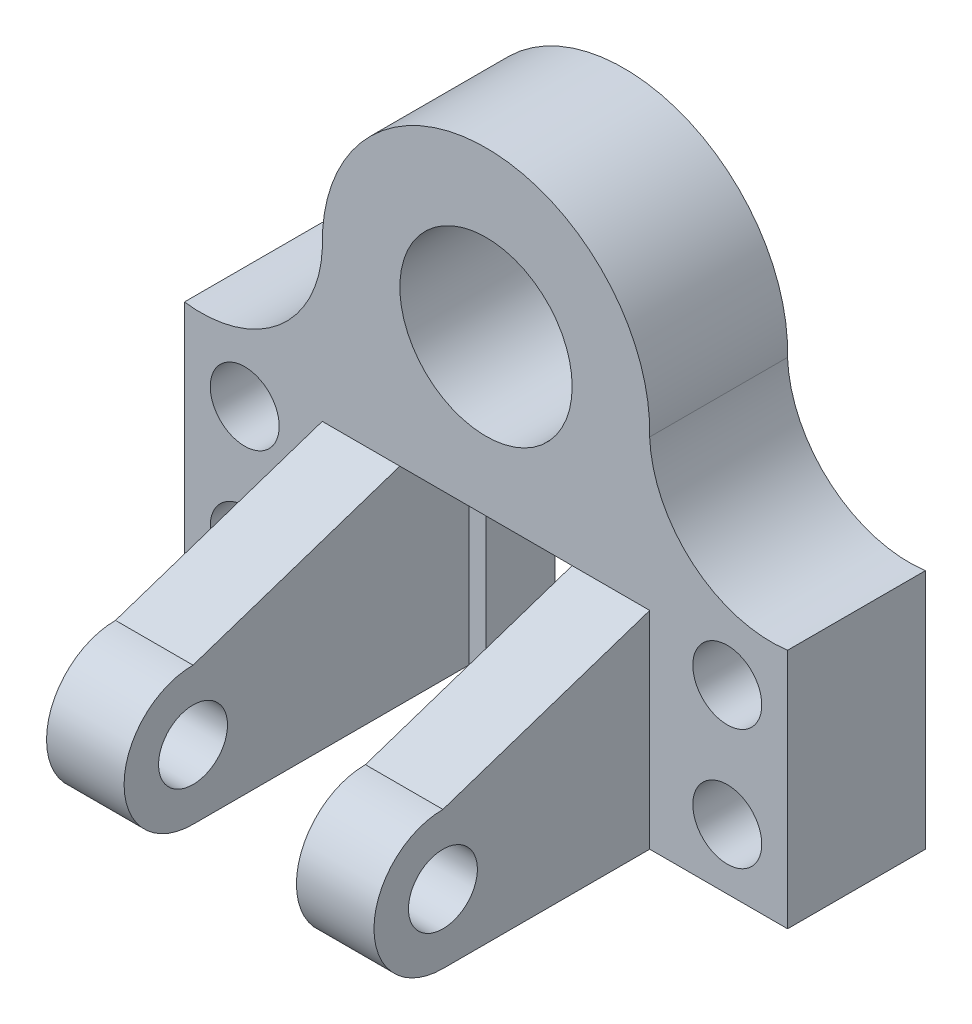
ISO-10303-21;
HEADER;
FILE_DESCRIPTION(('STEP AP214'),'2;1');
FILE_NAME('part.step','',(''),(''),'','','');
FILE_SCHEMA(('AUTOMOTIVE_DESIGN { 1 0 10303 214 1 1 1 1 }'));
ENDSEC;
DATA;
#1=APPLICATION_CONTEXT('core data for automotive mechanical design processes');
#2=APPLICATION_PROTOCOL_DEFINITION('international standard','automotive_design',2000,#1);
#3=PRODUCT_CONTEXT('',#1,'mechanical');
#4=PRODUCT('Part','Part','',(#3));
#5=PRODUCT_RELATED_PRODUCT_CATEGORY('part','',(#4));
#6=PRODUCT_DEFINITION_FORMATION('','',#4);
#7=PRODUCT_DEFINITION_CONTEXT('part definition',#1,'design');
#8=PRODUCT_DEFINITION('design','',#6,#7);
#9=PRODUCT_DEFINITION_SHAPE('','',#8);
#10=(LENGTH_UNIT() NAMED_UNIT(*) SI_UNIT(.MILLI.,.METRE.));
#11=(NAMED_UNIT(*) PLANE_ANGLE_UNIT() SI_UNIT($,.RADIAN.));
#12=(NAMED_UNIT(*) SI_UNIT($,.STERADIAN.) SOLID_ANGLE_UNIT());
#13=UNCERTAINTY_MEASURE_WITH_UNIT(LENGTH_MEASURE(1.E-05),#10,'distance_accuracy_value','');
#14=(GEOMETRIC_REPRESENTATION_CONTEXT(3) GLOBAL_UNCERTAINTY_ASSIGNED_CONTEXT((#13)) GLOBAL_UNIT_ASSIGNED_CONTEXT((#10,
#11,#12)) REPRESENTATION_CONTEXT('',''));
#15=CARTESIAN_POINT('',(0.,0.,0.));
#16=DIRECTION('',(0.,0.,1.));
#17=DIRECTION('',(1.,0.,0.));
#18=AXIS2_PLACEMENT_3D('',#15,#16,#17);
#19=CARTESIAN_POINT('',(38.,16.,64.));
#20=DIRECTION('',(-1.,0.,0.));
#21=DIRECTION('',(0.,-1.,0.));
#22=AXIS2_PLACEMENT_3D('',#19,#20,#21);
#23=CYLINDRICAL_SURFACE('',#22,8.00000000000001);
#24=CARTESIAN_POINT('',(-38.,16.,64.));
#25=DIRECTION('',(-1.,0.,0.));
#26=DIRECTION('',(0.,-1.,0.));
#27=AXIS2_PLACEMENT_3D('',#24,#25,#26);
#28=CIRCLE('',#27,8.00000000000001);
#29=CARTESIAN_POINT('',(-38.,7.99999999999998,64.));
#30=VERTEX_POINT('',#29);
#31=EDGE_CURVE('E244',#30,#30,#28,.T.);
#32=ORIENTED_EDGE('',*,*,#31,.T.);
#33=EDGE_LOOP('',(#32));
#34=FACE_BOUND('',#33,.T.);
#35=CARTESIAN_POINT('',(-20.,16.,64.));
#36=DIRECTION('',(1.,0.,0.));
#37=DIRECTION('',(0.,1.,0.));
#38=AXIS2_PLACEMENT_3D('',#35,#36,#37);
#39=CIRCLE('',#38,8.00000000000001);
#40=CARTESIAN_POINT('',(-20.,24.,64.));
#41=VERTEX_POINT('',#40);
#42=EDGE_CURVE('E215',#41,#41,#39,.F.);
#43=ORIENTED_EDGE('',*,*,#42,.F.);
#44=EDGE_LOOP('',(#43));
#45=FACE_BOUND('',#44,.T.);
#46=ADVANCED_FACE('F41',(#34,#45),#23,.F.);
#47=CARTESIAN_POINT('',(38.,16.,64.));
#48=DIRECTION('',(-1.,0.,0.));
#49=DIRECTION('',(0.,-1.,0.));
#50=AXIS2_PLACEMENT_3D('',#47,#48,#49);
#51=CYLINDRICAL_SURFACE('',#50,16.);
#52=DIRECTION('',(1.,0.,0.));
#53=VECTOR('',#52,1.);
#54=CARTESIAN_POINT('',(0.,0.,64.));
#55=LINE('',#54,#53);
#56=CARTESIAN_POINT('',(-38.,0.,64.));
#57=VERTEX_POINT('',#56);
#58=CARTESIAN_POINT('',(-20.,0.,64.));
#59=VERTEX_POINT('',#58);
#60=EDGE_CURVE('E270',#57,#59,#55,.T.);
#61=ORIENTED_EDGE('',*,*,#60,.T.);
#62=CARTESIAN_POINT('',(-20.,16.,64.));
#63=DIRECTION('',(1.,0.,0.));
#64=DIRECTION('',(0.,1.,0.));
#65=AXIS2_PLACEMENT_3D('',#62,#63,#64);
#66=CIRCLE('',#65,16.);
#67=CARTESIAN_POINT('',(-20.,32.,64.));
#68=VERTEX_POINT('',#67);
#69=EDGE_CURVE('E184',#59,#68,#66,.F.);
#70=ORIENTED_EDGE('',*,*,#69,.T.);
#71=DIRECTION('',(-1.,0.,0.));
#72=VECTOR('',#71,1.);
#73=CARTESIAN_POINT('',(38.,32.,64.));
#74=LINE('',#73,#72);
#75=CARTESIAN_POINT('',(-38.,32.,64.));
#76=VERTEX_POINT('',#75);
#77=EDGE_CURVE('E254',#68,#76,#74,.T.);
#78=ORIENTED_EDGE('',*,*,#77,.T.);
#79=CARTESIAN_POINT('',(-38.,16.,64.));
#80=DIRECTION('',(-1.,0.,0.));
#81=DIRECTION('',(0.,-1.,0.));
#82=AXIS2_PLACEMENT_3D('',#79,#80,#81);
#83=CIRCLE('',#82,16.);
#84=EDGE_CURVE('E249',#57,#76,#83,.T.);
#85=ORIENTED_EDGE('',*,*,#84,.F.);
#86=EDGE_LOOP('',(#61,#70,#78,#85));
#87=FACE_BOUND('',#86,.T.);
#88=ADVANCED_FACE('F427',(#87),#51,.T.);
#89=CARTESIAN_POINT('',(0.,0.,16.));
#90=DIRECTION('',(0.,1.,0.));
#91=DIRECTION('',(-1.,0.,0.));
#92=AXIS2_PLACEMENT_3D('',#89,#90,#91);
#93=PLANE('',#92);
#94=DIRECTION('',(1.,0.,0.));
#95=VECTOR('',#94,1.);
#96=CARTESIAN_POINT('',(0.,0.,0.));
#97=LINE('',#96,#95);
#98=CARTESIAN_POINT('',(-20.,0.,0.));
#99=VERTEX_POINT('',#98);
#100=CARTESIAN_POINT('',(-16.,0.,0.));
#101=VERTEX_POINT('',#100);
#102=EDGE_CURVE('E57',#99,#101,#97,.T.);
#103=ORIENTED_EDGE('',*,*,#102,.F.);
#104=DIRECTION('',(0.,0.,-1.));
#105=VECTOR('',#104,1.);
#106=CARTESIAN_POINT('',(-20.,0.,64.));
#107=LINE('',#106,#105);
#108=EDGE_CURVE('E195',#59,#99,#107,.T.);
#109=ORIENTED_EDGE('',*,*,#108,.F.);
#110=ORIENTED_EDGE('',*,*,#60,.F.);
#111=DIRECTION('',(0.,0.,-1.));
#112=VECTOR('',#111,1.);
#113=CARTESIAN_POINT('',(-38.,0.,64.));
#114=LINE('',#113,#112);
#115=CARTESIAN_POINT('',(-38.,0.,16.));
#116=VERTEX_POINT('',#115);
#117=EDGE_CURVE('E275',#57,#116,#114,.T.);
#118=ORIENTED_EDGE('',*,*,#117,.T.);
#119=DIRECTION('',(1.,0.,0.));
#120=VECTOR('',#119,1.);
#121=CARTESIAN_POINT('',(0.,0.,16.));
#122=LINE('',#121,#120);
#123=CARTESIAN_POINT('',(-70.,0.,16.));
#124=VERTEX_POINT('',#123);
#125=EDGE_CURVE('E286',#124,#116,#122,.T.);
#126=ORIENTED_EDGE('',*,*,#125,.F.);
#127=DIRECTION('',(0.,0.,-1.));
#128=VECTOR('',#127,1.);
#129=CARTESIAN_POINT('',(-70.,0.,16.));
#130=LINE('',#129,#128);
#131=CARTESIAN_POINT('',(-70.,0.,-16.));
#132=VERTEX_POINT('',#131);
#133=EDGE_CURVE('E352',#124,#132,#130,.T.);
#134=ORIENTED_EDGE('',*,*,#133,.T.);
#135=DIRECTION('',(1.,0.,0.));
#136=VECTOR('',#135,1.);
#137=CARTESIAN_POINT('',(0.,0.,-16.));
#138=LINE('',#137,#136);
#139=CARTESIAN_POINT('',(-16.,0.,-16.));
#140=VERTEX_POINT('',#139);
#141=EDGE_CURVE('E330',#132,#140,#138,.T.);
#142=ORIENTED_EDGE('',*,*,#141,.T.);
#143=DIRECTION('',(0.,0.,-1.));
#144=VECTOR('',#143,1.);
#145=CARTESIAN_POINT('',(-16.,0.,16.));
#146=LINE('',#145,#144);
#147=EDGE_CURVE('E235',#101,#140,#146,.T.);
#148=ORIENTED_EDGE('',*,*,#147,.F.);
#149=EDGE_LOOP('',(#103,#109,#110,#118,#126,#134,#142,#148));
#150=FACE_BOUND('',#149,.T.);
#151=ADVANCED_FACE('F395',(#150),#93,.F.);
#152=CARTESIAN_POINT('',(-16.,0.,16.));
#153=DIRECTION('',(1.,0.,0.));
#154=DIRECTION('',(0.,0.,-1.));
#155=AXIS2_PLACEMENT_3D('',#152,#153,#154);
#156=PLANE('',#155);
#157=DIRECTION('',(0.,0.,-1.));
#158=VECTOR('',#157,1.);
#159=CARTESIAN_POINT('',(-16.,48.,16.));
#160=LINE('',#159,#158);
#161=CARTESIAN_POINT('',(-16.,48.,0.));
#162=VERTEX_POINT('',#161);
#163=CARTESIAN_POINT('',(-16.,48.,-16.));
#164=VERTEX_POINT('',#163);
#165=EDGE_CURVE('E229',#162,#164,#160,.T.);
#166=ORIENTED_EDGE('',*,*,#165,.F.);
#167=DIRECTION('',(0.,-1.,0.));
#168=VECTOR('',#167,1.);
#169=CARTESIAN_POINT('',(-16.,0.,0.));
#170=LINE('',#169,#168);
#171=EDGE_CURVE('E187',#162,#101,#170,.T.);
#172=ORIENTED_EDGE('',*,*,#171,.T.);
#173=ORIENTED_EDGE('',*,*,#147,.T.);
#174=DIRECTION('',(0.,-1.,0.));
#175=VECTOR('',#174,1.);
#176=CARTESIAN_POINT('',(-16.,0.,-16.));
#177=LINE('',#176,#175);
#178=EDGE_CURVE('E227',#164,#140,#177,.T.);
#179=ORIENTED_EDGE('',*,*,#178,.F.);
#180=EDGE_LOOP('',(#166,#172,#173,#179));
#181=FACE_BOUND('',#180,.T.);
#182=ADVANCED_FACE('F386',(#181),#156,.T.);
#183=CARTESIAN_POINT('',(16.,0.,16.));
#184=DIRECTION('',(1.,0.,0.));
#185=DIRECTION('',(0.,0.,-1.));
#186=AXIS2_PLACEMENT_3D('',#183,#184,#185);
#187=PLANE('',#186);
#188=DIRECTION('',(0.,-1.,0.));
#189=VECTOR('',#188,1.);
#190=CARTESIAN_POINT('',(16.,0.,0.));
#191=LINE('',#190,#189);
#192=CARTESIAN_POINT('',(16.,48.,0.));
#193=VERTEX_POINT('',#192);
#194=CARTESIAN_POINT('',(16.,0.,0.));
#195=VERTEX_POINT('',#194);
#196=EDGE_CURVE('E203',#193,#195,#191,.T.);
#197=ORIENTED_EDGE('',*,*,#196,.F.);
#198=DIRECTION('',(0.,0.,-1.));
#199=VECTOR('',#198,1.);
#200=CARTESIAN_POINT('',(16.,48.,16.));
#201=LINE('',#200,#199);
#202=CARTESIAN_POINT('',(16.,48.,-16.));
#203=VERTEX_POINT('',#202);
#204=EDGE_CURVE('E222',#193,#203,#201,.T.);
#205=ORIENTED_EDGE('',*,*,#204,.T.);
#206=DIRECTION('',(0.,-1.,0.));
#207=VECTOR('',#206,1.);
#208=CARTESIAN_POINT('',(16.,0.,-16.));
#209=LINE('',#208,#207);
#210=CARTESIAN_POINT('',(16.,0.,-16.));
#211=VERTEX_POINT('',#210);
#212=EDGE_CURVE('E219',#203,#211,#209,.T.);
#213=ORIENTED_EDGE('',*,*,#212,.T.);
#214=DIRECTION('',(0.,0.,-1.));
#215=VECTOR('',#214,1.);
#216=CARTESIAN_POINT('',(16.,0.,16.));
#217=LINE('',#216,#215);
#218=EDGE_CURVE('E225',#195,#211,#217,.T.);
#219=ORIENTED_EDGE('',*,*,#218,.F.);
#220=EDGE_LOOP('',(#197,#205,#213,#219));
#221=FACE_BOUND('',#220,.T.);
#222=ADVANCED_FACE('F381',(#221),#187,.F.);
#223=CARTESIAN_POINT('',(0.,48.,16.));
#224=DIRECTION('',(0.,-1.,0.));
#225=DIRECTION('',(0.,0.,-1.));
#226=AXIS2_PLACEMENT_3D('',#223,#224,#225);
#227=PLANE('',#226);
#228=DIRECTION('',(-1.,0.,0.));
#229=VECTOR('',#228,1.);
#230=CARTESIAN_POINT('',(0.,48.,-16.));
#231=LINE('',#230,#229);
#232=EDGE_CURVE('E329',#203,#164,#231,.T.);
#233=ORIENTED_EDGE('',*,*,#232,.F.);
#234=ORIENTED_EDGE('',*,*,#204,.F.);
#235=DIRECTION('',(1.,0.,0.));
#236=VECTOR('',#235,1.);
#237=CARTESIAN_POINT('',(0.,48.,0.));
#238=LINE('',#237,#236);
#239=CARTESIAN_POINT('',(20.,48.,0.));
#240=VERTEX_POINT('',#239);
#241=EDGE_CURVE('E61',#193,#240,#238,.T.);
#242=ORIENTED_EDGE('',*,*,#241,.T.);
#243=DIRECTION('',(0.,0.,-1.));
#244=VECTOR('',#243,1.);
#245=CARTESIAN_POINT('',(20.,48.,147.));
#246=LINE('',#245,#244);
#247=CARTESIAN_POINT('',(20.,47.9999999999999,16.0000000000005));
#248=VERTEX_POINT('',#247);
#249=EDGE_CURVE('E198',#248,#240,#246,.T.);
#250=ORIENTED_EDGE('',*,*,#249,.F.);
#251=DIRECTION('',(-1.,0.,0.));
#252=VECTOR('',#251,1.);
#253=CARTESIAN_POINT('',(0.,48.,16.));
#254=LINE('',#253,#252);
#255=CARTESIAN_POINT('',(-20.,47.9999999999999,16.0000000000005));
#256=VERTEX_POINT('',#255);
#257=EDGE_CURVE('E181',#248,#256,#254,.T.);
#258=ORIENTED_EDGE('',*,*,#257,.T.);
#259=DIRECTION('',(0.,0.,-1.));
#260=VECTOR('',#259,1.);
#261=CARTESIAN_POINT('',(-20.,48.,147.));
#262=LINE('',#261,#260);
#263=CARTESIAN_POINT('',(-20.,48.,0.));
#264=VERTEX_POINT('',#263);
#265=EDGE_CURVE('E172',#256,#264,#262,.T.);
#266=ORIENTED_EDGE('',*,*,#265,.T.);
#267=DIRECTION('',(1.,0.,0.));
#268=VECTOR('',#267,1.);
#269=CARTESIAN_POINT('',(0.,48.,0.));
#270=LINE('',#269,#268);
#271=EDGE_CURVE('E177',#264,#162,#270,.T.);
#272=ORIENTED_EDGE('',*,*,#271,.T.);
#273=ORIENTED_EDGE('',*,*,#165,.T.);
#274=EDGE_LOOP('',(#233,#234,#242,#250,#258,#266,#272,#273));
#275=FACE_BOUND('',#274,.T.);
#276=ADVANCED_FACE('F180',(#275),#227,.T.);
#277=CARTESIAN_POINT('',(-38.,0.,64.));
#278=DIRECTION('',(1.,0.,0.));
#279=DIRECTION('',(0.,1.,0.));
#280=AXIS2_PLACEMENT_3D('',#277,#278,#279);
#281=PLANE('',#280);
#282=ORIENTED_EDGE('',*,*,#31,.F.);
#283=EDGE_LOOP('',(#282));
#284=FACE_BOUND('',#283,.T.);
#285=DIRECTION('',(0.,0.316227766016838,-0.948683298050514));
#286=VECTOR('',#285,1.);
#287=CARTESIAN_POINT('',(-38.,48.,16.));
#288=LINE('',#287,#286);
#289=CARTESIAN_POINT('',(-38.,48.,16.));
#290=VERTEX_POINT('',#289);
#291=EDGE_CURVE('E234',#76,#290,#288,.T.);
#292=ORIENTED_EDGE('',*,*,#291,.T.);
#293=DIRECTION('',(0.,-1.,0.));
#294=VECTOR('',#293,1.);
#295=CARTESIAN_POINT('',(-38.,0.,16.));
#296=LINE('',#295,#294);
#297=EDGE_CURVE('E288',#290,#116,#296,.T.);
#298=ORIENTED_EDGE('',*,*,#297,.T.);
#299=ORIENTED_EDGE('',*,*,#117,.F.);
#300=ORIENTED_EDGE('',*,*,#84,.T.);
#301=EDGE_LOOP('',(#292,#298,#299,#300));
#302=FACE_BOUND('',#301,.T.);
#303=ADVANCED_FACE('F494',(#284,#302),#281,.F.);
#304=CARTESIAN_POINT('',(-20.,0.,64.));
#305=DIRECTION('',(1.,0.,0.));
#306=DIRECTION('',(0.,1.,0.));
#307=AXIS2_PLACEMENT_3D('',#304,#305,#306);
#308=PLANE('',#307);
#309=ORIENTED_EDGE('',*,*,#108,.T.);
#310=DIRECTION('',(0.,-1.,0.));
#311=VECTOR('',#310,1.);
#312=CARTESIAN_POINT('',(-20.,0.,0.));
#313=LINE('',#312,#311);
#314=EDGE_CURVE('E189',#264,#99,#313,.T.);
#315=ORIENTED_EDGE('',*,*,#314,.F.);
#316=ORIENTED_EDGE('',*,*,#265,.F.);
#317=DIRECTION('',(0.,-0.316227766016838,0.948683298050514));
#318=VECTOR('',#317,1.);
#319=CARTESIAN_POINT('',(-20.,28.8,73.6));
#320=LINE('',#319,#318);
#321=EDGE_CURVE('E243',#256,#68,#320,.T.);
#322=ORIENTED_EDGE('',*,*,#321,.T.);
#323=ORIENTED_EDGE('',*,*,#69,.F.);
#324=EDGE_LOOP('',(#309,#315,#316,#322,#323));
#325=FACE_BOUND('',#324,.T.);
#326=ORIENTED_EDGE('',*,*,#42,.T.);
#327=EDGE_LOOP('',(#326));
#328=FACE_BOUND('',#327,.T.);
#329=ADVANCED_FACE('F186',(#325,#328),#308,.T.);
#330=CARTESIAN_POINT('',(38.,0.,64.));
#331=DIRECTION('',(1.,0.,0.));
#332=DIRECTION('',(0.,1.,0.));
#333=AXIS2_PLACEMENT_3D('',#330,#331,#332);
#334=PLANE('',#333);
#335=CARTESIAN_POINT('',(38.,16.,64.));
#336=DIRECTION('',(-1.,0.,0.));
#337=DIRECTION('',(0.,-1.,0.));
#338=AXIS2_PLACEMENT_3D('',#335,#336,#337);
#339=CIRCLE('',#338,8.00000000000001);
#340=CARTESIAN_POINT('',(38.,7.99999999999999,64.));
#341=VERTEX_POINT('',#340);
#342=EDGE_CURVE('E246',#341,#341,#339,.T.);
#343=ORIENTED_EDGE('',*,*,#342,.T.);
#344=EDGE_LOOP('',(#343));
#345=FACE_BOUND('',#344,.T.);
#346=DIRECTION('',(0.,-1.,0.));
#347=VECTOR('',#346,1.);
#348=CARTESIAN_POINT('',(38.,0.,16.));
#349=LINE('',#348,#347);
#350=CARTESIAN_POINT('',(38.,48.,16.));
#351=VERTEX_POINT('',#350);
#352=CARTESIAN_POINT('',(38.,0.,16.));
#353=VERTEX_POINT('',#352);
#354=EDGE_CURVE('E300',#351,#353,#349,.T.);
#355=ORIENTED_EDGE('',*,*,#354,.F.);
#356=DIRECTION('',(0.,-0.316227766016838,0.948683298050514));
#357=VECTOR('',#356,1.);
#358=CARTESIAN_POINT('',(38.,28.8,73.6));
#359=LINE('',#358,#357);
#360=CARTESIAN_POINT('',(38.,32.,64.));
#361=VERTEX_POINT('',#360);
#362=EDGE_CURVE('E239',#351,#361,#359,.T.);
#363=ORIENTED_EDGE('',*,*,#362,.T.);
#364=CARTESIAN_POINT('',(38.,16.,64.));
#365=DIRECTION('',(-1.,0.,0.));
#366=DIRECTION('',(0.,-1.,0.));
#367=AXIS2_PLACEMENT_3D('',#364,#365,#366);
#368=CIRCLE('',#367,16.);
#369=CARTESIAN_POINT('',(38.,0.,64.));
#370=VERTEX_POINT('',#369);
#371=EDGE_CURVE('E248',#370,#361,#368,.T.);
#372=ORIENTED_EDGE('',*,*,#371,.F.);
#373=DIRECTION('',(0.,0.,-1.));
#374=VECTOR('',#373,1.);
#375=CARTESIAN_POINT('',(38.,0.,64.));
#376=LINE('',#375,#374);
#377=EDGE_CURVE('E261',#370,#353,#376,.T.);
#378=ORIENTED_EDGE('',*,*,#377,.T.);
#379=EDGE_LOOP('',(#355,#363,#372,#378));
#380=FACE_BOUND('',#379,.T.);
#381=ADVANCED_FACE('F458',(#345,#380),#334,.T.);
#382=CARTESIAN_POINT('',(20.,0.,64.));
#383=DIRECTION('',(1.,0.,0.));
#384=DIRECTION('',(0.,0.,-1.));
#385=AXIS2_PLACEMENT_3D('',#382,#383,#384);
#386=PLANE('',#385);
#387=DIRECTION('',(0.,-0.316227766016838,0.948683298050514));
#388=VECTOR('',#387,1.);
#389=CARTESIAN_POINT('',(20.,28.8,73.6));
#390=LINE('',#389,#388);
#391=CARTESIAN_POINT('',(20.,32.,64.));
#392=VERTEX_POINT('',#391);
#393=EDGE_CURVE('E240',#248,#392,#390,.T.);
#394=ORIENTED_EDGE('',*,*,#393,.F.);
#395=ORIENTED_EDGE('',*,*,#249,.T.);
#396=DIRECTION('',(0.,-1.,0.));
#397=VECTOR('',#396,1.);
#398=CARTESIAN_POINT('',(20.,0.,0.));
#399=LINE('',#398,#397);
#400=CARTESIAN_POINT('',(20.,0.,0.));
#401=VERTEX_POINT('',#400);
#402=EDGE_CURVE('E196',#240,#401,#399,.T.);
#403=ORIENTED_EDGE('',*,*,#402,.T.);
#404=DIRECTION('',(0.,0.,-1.));
#405=VECTOR('',#404,1.);
#406=CARTESIAN_POINT('',(20.,0.,64.));
#407=LINE('',#406,#405);
#408=CARTESIAN_POINT('',(20.,0.,64.));
#409=VERTEX_POINT('',#408);
#410=EDGE_CURVE('E269',#409,#401,#407,.T.);
#411=ORIENTED_EDGE('',*,*,#410,.F.);
#412=CARTESIAN_POINT('',(20.,16.,64.));
#413=DIRECTION('',(1.,0.,0.));
#414=DIRECTION('',(0.,0.,-1.));
#415=AXIS2_PLACEMENT_3D('',#412,#413,#414);
#416=CIRCLE('',#415,16.);
#417=EDGE_CURVE('E213',#409,#392,#416,.F.);
#418=ORIENTED_EDGE('',*,*,#417,.T.);
#419=EDGE_LOOP('',(#394,#395,#403,#411,#418));
#420=FACE_BOUND('',#419,.T.);
#421=CARTESIAN_POINT('',(20.,16.,64.));
#422=DIRECTION('',(1.,0.,0.));
#423=DIRECTION('',(0.,0.,-1.));
#424=AXIS2_PLACEMENT_3D('',#421,#422,#423);
#425=CIRCLE('',#424,8.00000000000001);
#426=CARTESIAN_POINT('',(20.,16.,56.));
#427=VERTEX_POINT('',#426);
#428=EDGE_CURVE('E220',#427,#427,#425,.F.);
#429=ORIENTED_EDGE('',*,*,#428,.F.);
#430=EDGE_LOOP('',(#429));
#431=FACE_BOUND('',#430,.T.);
#432=ADVANCED_FACE('F457',(#420,#431),#386,.F.);
#433=CARTESIAN_POINT('',(66.2094033057084,83.9945329788019,16.));
#434=DIRECTION('',(0.,0.,-1.));
#435=DIRECTION('',(-1.,0.,0.));
#436=AXIS2_PLACEMENT_3D('',#433,#434,#435);
#437=CYLINDRICAL_SURFACE('',#436,28.25);
#438=CARTESIAN_POINT('',(66.2094033057084,83.9945329788019,-16.));
#439=DIRECTION('',(0.,0.,1.));
#440=DIRECTION('',(1.,0.,0.));
#441=AXIS2_PLACEMENT_3D('',#438,#439,#440);
#442=CIRCLE('',#441,28.25);
#443=CARTESIAN_POINT('',(37.9825960604593,82.8500449974093,-16.));
#444=VERTEX_POINT('',#443);
#445=CARTESIAN_POINT('',(70.,56.,-16.));
#446=VERTEX_POINT('',#445);
#447=EDGE_CURVE('E273',#444,#446,#442,.T.);
#448=ORIENTED_EDGE('',*,*,#447,.F.);
#449=DIRECTION('',(0.,0.,-1.));
#450=VECTOR('',#449,1.);
#451=CARTESIAN_POINT('',(37.9825960604593,82.8500449974093,16.));
#452=LINE('',#451,#450);
#453=CARTESIAN_POINT('',(37.9825960604593,82.8500449974093,16.));
#454=VERTEX_POINT('',#453);
#455=EDGE_CURVE('E47',#454,#444,#452,.T.);
#456=ORIENTED_EDGE('',*,*,#455,.F.);
#457=CARTESIAN_POINT('',(66.2094033057084,83.9945329788019,16.));
#458=DIRECTION('',(0.,0.,1.));
#459=DIRECTION('',(1.,0.,0.));
#460=AXIS2_PLACEMENT_3D('',#457,#458,#459);
#461=CIRCLE('',#460,28.25);
#462=CARTESIAN_POINT('',(70.,56.,16.));
#463=VERTEX_POINT('',#462);
#464=EDGE_CURVE('E277',#454,#463,#461,.T.);
#465=ORIENTED_EDGE('',*,*,#464,.T.);
#466=DIRECTION('',(0.,0.,-1.));
#467=VECTOR('',#466,1.);
#468=CARTESIAN_POINT('',(70.,56.,16.));
#469=LINE('',#468,#467);
#470=EDGE_CURVE('E317',#463,#446,#469,.T.);
#471=ORIENTED_EDGE('',*,*,#470,.T.);
#472=EDGE_LOOP('',(#448,#456,#465,#471));
#473=FACE_BOUND('',#472,.T.);
#474=ADVANCED_FACE('F43',(#473),#437,.F.);
#475=CARTESIAN_POINT('',(0.,84.,16.));
#476=DIRECTION('',(0.,0.,-1.));
#477=DIRECTION('',(-1.,0.,0.));
#478=AXIS2_PLACEMENT_3D('',#475,#476,#477);
#479=CYLINDRICAL_SURFACE('',#478,38.);
#480=CARTESIAN_POINT('',(0.,84.,-16.));
#481=DIRECTION('',(0.,0.,1.));
#482=DIRECTION('',(1.,0.,0.));
#483=AXIS2_PLACEMENT_3D('',#480,#481,#482);
#484=CIRCLE('',#483,38.);
#485=CARTESIAN_POINT('',(-37.9825960604593,82.8500449974094,-16.));
#486=VERTEX_POINT('',#485);
#487=EDGE_CURVE('E316',#444,#486,#484,.T.);
#488=ORIENTED_EDGE('',*,*,#487,.T.);
#489=DIRECTION('',(0.,0.,-1.));
#490=VECTOR('',#489,1.);
#491=CARTESIAN_POINT('',(-37.9825960604593,82.8500449974094,16.));
#492=LINE('',#491,#490);
#493=CARTESIAN_POINT('',(-37.9825960604593,82.8500449974094,16.));
#494=VERTEX_POINT('',#493);
#495=EDGE_CURVE('E360',#494,#486,#492,.T.);
#496=ORIENTED_EDGE('',*,*,#495,.F.);
#497=CARTESIAN_POINT('',(0.,84.,16.));
#498=DIRECTION('',(0.,0.,1.));
#499=DIRECTION('',(1.,0.,0.));
#500=AXIS2_PLACEMENT_3D('',#497,#498,#499);
#501=CIRCLE('',#500,38.);
#502=EDGE_CURVE('E276',#454,#494,#501,.T.);
#503=ORIENTED_EDGE('',*,*,#502,.F.);
#504=ORIENTED_EDGE('',*,*,#455,.T.);
#505=EDGE_LOOP('',(#488,#496,#503,#504));
#506=FACE_BOUND('',#505,.T.);
#507=ADVANCED_FACE('F364',(#506),#479,.T.);
#508=CARTESIAN_POINT('',(-66.2094033057084,83.9945329788019,16.));
#509=DIRECTION('',(0.,0.,-1.));
#510=DIRECTION('',(-1.,0.,0.));
#511=AXIS2_PLACEMENT_3D('',#508,#509,#510);
#512=CYLINDRICAL_SURFACE('',#511,28.25);
#513=CARTESIAN_POINT('',(-66.2094033057084,83.9945329788019,-16.));
#514=DIRECTION('',(0.,0.,1.));
#515=DIRECTION('',(1.,0.,0.));
#516=AXIS2_PLACEMENT_3D('',#513,#514,#515);
#517=CIRCLE('',#516,28.25);
#518=CARTESIAN_POINT('',(-70.,56.,-16.));
#519=VERTEX_POINT('',#518);
#520=EDGE_CURVE('E322',#486,#519,#517,.F.);
#521=ORIENTED_EDGE('',*,*,#520,.T.);
#522=DIRECTION('',(0.,0.,-1.));
#523=VECTOR('',#522,1.);
#524=CARTESIAN_POINT('',(-70.,56.,16.));
#525=LINE('',#524,#523);
#526=CARTESIAN_POINT('',(-70.,56.,16.));
#527=VERTEX_POINT('',#526);
#528=EDGE_CURVE('E357',#527,#519,#525,.T.);
#529=ORIENTED_EDGE('',*,*,#528,.F.);
#530=CARTESIAN_POINT('',(-66.2094033057084,83.9945329788019,16.));
#531=DIRECTION('',(0.,0.,1.));
#532=DIRECTION('',(1.,0.,0.));
#533=AXIS2_PLACEMENT_3D('',#530,#531,#532);
#534=CIRCLE('',#533,28.25);
#535=EDGE_CURVE('E285',#494,#527,#534,.F.);
#536=ORIENTED_EDGE('',*,*,#535,.F.);
#537=ORIENTED_EDGE('',*,*,#495,.T.);
#538=EDGE_LOOP('',(#521,#529,#536,#537));
#539=FACE_BOUND('',#538,.T.);
#540=ADVANCED_FACE('F402',(#539),#512,.F.);
#541=CARTESIAN_POINT('',(-70.,0.,16.));
#542=DIRECTION('',(-1.,0.,0.));
#543=DIRECTION('',(0.,0.,1.));
#544=AXIS2_PLACEMENT_3D('',#541,#542,#543);
#545=PLANE('',#544);
#546=DIRECTION('',(0.,1.,0.));
#547=VECTOR('',#546,1.);
#548=CARTESIAN_POINT('',(-70.,0.,-16.));
#549=LINE('',#548,#547);
#550=EDGE_CURVE('E321',#132,#519,#549,.T.);
#551=ORIENTED_EDGE('',*,*,#550,.F.);
#552=ORIENTED_EDGE('',*,*,#133,.F.);
#553=DIRECTION('',(0.,1.,0.));
#554=VECTOR('',#553,1.);
#555=CARTESIAN_POINT('',(-70.,0.,16.));
#556=LINE('',#555,#554);
#557=EDGE_CURVE('E282',#124,#527,#556,.T.);
#558=ORIENTED_EDGE('',*,*,#557,.T.);
#559=ORIENTED_EDGE('',*,*,#528,.T.);
#560=EDGE_LOOP('',(#551,#552,#558,#559));
#561=FACE_BOUND('',#560,.T.);
#562=ADVANCED_FACE('F399',(#561),#545,.T.);
#563=ORIENTED_EDGE('',*,*,#410,.T.);
#564=DIRECTION('',(1.,0.,0.));
#565=VECTOR('',#564,1.);
#566=CARTESIAN_POINT('',(0.,0.,0.));
#567=LINE('',#566,#565);
#568=EDGE_CURVE('E207',#195,#401,#567,.T.);
#569=ORIENTED_EDGE('',*,*,#568,.F.);
#570=ORIENTED_EDGE('',*,*,#218,.T.);
#571=CARTESIAN_POINT('',(70.,0.,-16.));
#572=VERTEX_POINT('',#571);
#573=EDGE_CURVE('E334',#211,#572,#138,.T.);
#574=ORIENTED_EDGE('',*,*,#573,.T.);
#575=DIRECTION('',(0.,0.,-1.));
#576=VECTOR('',#575,1.);
#577=CARTESIAN_POINT('',(70.,0.,16.));
#578=LINE('',#577,#576);
#579=CARTESIAN_POINT('',(70.,0.,16.));
#580=VERTEX_POINT('',#579);
#581=EDGE_CURVE('E351',#580,#572,#578,.T.);
#582=ORIENTED_EDGE('',*,*,#581,.F.);
#583=EDGE_CURVE('E287',#353,#580,#122,.T.);
#584=ORIENTED_EDGE('',*,*,#583,.F.);
#585=ORIENTED_EDGE('',*,*,#377,.F.);
#586=DIRECTION('',(1.,0.,0.));
#587=VECTOR('',#586,1.);
#588=CARTESIAN_POINT('',(0.,0.,64.));
#589=LINE('',#588,#587);
#590=EDGE_CURVE('E258',#409,#370,#589,.T.);
#591=ORIENTED_EDGE('',*,*,#590,.F.);
#592=EDGE_LOOP('',(#563,#569,#570,#574,#582,#584,#585,#591));
#593=FACE_BOUND('',#592,.T.);
#594=ADVANCED_FACE('F408',(#593),#93,.F.);
#595=CARTESIAN_POINT('',(0.,84.,16.));
#596=DIRECTION('',(0.,0.,-1.));
#597=DIRECTION('',(-1.,0.,0.));
#598=AXIS2_PLACEMENT_3D('',#595,#596,#597);
#599=CYLINDRICAL_SURFACE('',#598,20.);
#600=CARTESIAN_POINT('',(0.,84.,16.));
#601=DIRECTION('',(0.,0.,1.));
#602=DIRECTION('',(1.,0.,0.));
#603=AXIS2_PLACEMENT_3D('',#600,#601,#602);
#604=CIRCLE('',#603,20.);
#605=CARTESIAN_POINT('',(20.,84.,16.));
#606=VERTEX_POINT('',#605);
#607=EDGE_CURVE('E309',#606,#606,#604,.T.);
#608=ORIENTED_EDGE('',*,*,#607,.T.);
#609=EDGE_LOOP('',(#608));
#610=FACE_BOUND('',#609,.T.);
#611=CARTESIAN_POINT('',(0.,84.,-16.));
#612=DIRECTION('',(0.,0.,1.));
#613=DIRECTION('',(1.,0.,0.));
#614=AXIS2_PLACEMENT_3D('',#611,#612,#613);
#615=CIRCLE('',#614,20.);
#616=CARTESIAN_POINT('',(20.,84.,-16.));
#617=VERTEX_POINT('',#616);
#618=EDGE_CURVE('E348',#617,#617,#615,.T.);
#619=ORIENTED_EDGE('',*,*,#618,.F.);
#620=EDGE_LOOP('',(#619));
#621=FACE_BOUND('',#620,.T.);
#622=ADVANCED_FACE('F414',(#610,#621),#599,.F.);
#623=CARTESIAN_POINT('',(56.,42.,16.));
#624=DIRECTION('',(0.,0.,-1.));
#625=DIRECTION('',(-1.,0.,0.));
#626=AXIS2_PLACEMENT_3D('',#623,#624,#625);
#627=CYLINDRICAL_SURFACE('',#626,8.00000000000001);
#628=CARTESIAN_POINT('',(56.,42.,16.));
#629=DIRECTION('',(0.,0.,1.));
#630=DIRECTION('',(1.,0.,0.));
#631=AXIS2_PLACEMENT_3D('',#628,#629,#630);
#632=CIRCLE('',#631,8.00000000000001);
#633=CARTESIAN_POINT('',(64.,42.,16.));
#634=VERTEX_POINT('',#633);
#635=EDGE_CURVE('E310',#634,#634,#632,.T.);
#636=ORIENTED_EDGE('',*,*,#635,.T.);
#637=EDGE_LOOP('',(#636));
#638=FACE_BOUND('',#637,.T.);
#639=CARTESIAN_POINT('',(56.,42.,-16.));
#640=DIRECTION('',(0.,0.,1.));
#641=DIRECTION('',(1.,0.,0.));
#642=AXIS2_PLACEMENT_3D('',#639,#640,#641);
#643=CIRCLE('',#642,8.00000000000001);
#644=CARTESIAN_POINT('',(64.,42.,-16.));
#645=VERTEX_POINT('',#644);
#646=EDGE_CURVE('E344',#645,#645,#643,.T.);
#647=ORIENTED_EDGE('',*,*,#646,.F.);
#648=EDGE_LOOP('',(#647));
#649=FACE_BOUND('',#648,.T.);
#650=ADVANCED_FACE('F422',(#638,#649),#627,.F.);
#651=CARTESIAN_POINT('',(56.,14.,16.));
#652=DIRECTION('',(0.,0.,-1.));
#653=DIRECTION('',(-1.,0.,0.));
#654=AXIS2_PLACEMENT_3D('',#651,#652,#653);
#655=CYLINDRICAL_SURFACE('',#654,8.00000000000001);
#656=CARTESIAN_POINT('',(56.,14.,16.));
#657=DIRECTION('',(0.,0.,1.));
#658=DIRECTION('',(1.,0.,0.));
#659=AXIS2_PLACEMENT_3D('',#656,#657,#658);
#660=CIRCLE('',#659,8.00000000000001);
#661=CARTESIAN_POINT('',(64.,14.,16.));
#662=VERTEX_POINT('',#661);
#663=EDGE_CURVE('E302',#662,#662,#660,.T.);
#664=ORIENTED_EDGE('',*,*,#663,.T.);
#665=EDGE_LOOP('',(#664));
#666=FACE_BOUND('',#665,.T.);
#667=CARTESIAN_POINT('',(56.,14.,-16.));
#668=DIRECTION('',(0.,0.,1.));
#669=DIRECTION('',(1.,0.,0.));
#670=AXIS2_PLACEMENT_3D('',#667,#668,#669);
#671=CIRCLE('',#670,8.00000000000001);
#672=CARTESIAN_POINT('',(64.,14.,-16.));
#673=VERTEX_POINT('',#672);
#674=EDGE_CURVE('E338',#673,#673,#671,.T.);
#675=ORIENTED_EDGE('',*,*,#674,.F.);
#676=EDGE_LOOP('',(#675));
#677=FACE_BOUND('',#676,.T.);
#678=ADVANCED_FACE('F575',(#666,#677),#655,.F.);
#679=CARTESIAN_POINT('',(-56.,14.,16.));
#680=DIRECTION('',(0.,0.,-1.));
#681=DIRECTION('',(-1.,0.,0.));
#682=AXIS2_PLACEMENT_3D('',#679,#680,#681);
#683=CYLINDRICAL_SURFACE('',#682,8.00000000000001);
#684=CARTESIAN_POINT('',(-56.,14.,16.));
#685=DIRECTION('',(0.,0.,1.));
#686=DIRECTION('',(1.,0.,0.));
#687=AXIS2_PLACEMENT_3D('',#684,#685,#686);
#688=CIRCLE('',#687,8.00000000000001);
#689=CARTESIAN_POINT('',(-48.,14.,16.));
#690=VERTEX_POINT('',#689);
#691=EDGE_CURVE('E301',#690,#690,#688,.F.);
#692=ORIENTED_EDGE('',*,*,#691,.F.);
#693=EDGE_LOOP('',(#692));
#694=FACE_BOUND('',#693,.T.);
#695=CARTESIAN_POINT('',(-56.,14.,-16.));
#696=DIRECTION('',(0.,0.,1.));
#697=DIRECTION('',(1.,0.,0.));
#698=AXIS2_PLACEMENT_3D('',#695,#696,#697);
#699=CIRCLE('',#698,8.00000000000001);
#700=CARTESIAN_POINT('',(-48.,14.,-16.));
#701=VERTEX_POINT('',#700);
#702=EDGE_CURVE('E340',#701,#701,#699,.F.);
#703=ORIENTED_EDGE('',*,*,#702,.T.);
#704=EDGE_LOOP('',(#703));
#705=FACE_BOUND('',#704,.T.);
#706=ADVANCED_FACE('F562',(#694,#705),#683,.F.);
#707=CARTESIAN_POINT('',(70.,0.,16.));
#708=DIRECTION('',(-1.,0.,0.));
#709=DIRECTION('',(0.,0.,1.));
#710=AXIS2_PLACEMENT_3D('',#707,#708,#709);
#711=PLANE('',#710);
#712=DIRECTION('',(0.,1.,0.));
#713=VECTOR('',#712,1.);
#714=CARTESIAN_POINT('',(70.,0.,-16.));
#715=LINE('',#714,#713);
#716=EDGE_CURVE('E333',#572,#446,#715,.T.);
#717=ORIENTED_EDGE('',*,*,#716,.T.);
#718=ORIENTED_EDGE('',*,*,#470,.F.);
#719=DIRECTION('',(0.,1.,0.));
#720=VECTOR('',#719,1.);
#721=CARTESIAN_POINT('',(70.,0.,16.));
#722=LINE('',#721,#720);
#723=EDGE_CURVE('E299',#580,#463,#722,.T.);
#724=ORIENTED_EDGE('',*,*,#723,.F.);
#725=ORIENTED_EDGE('',*,*,#581,.T.);
#726=EDGE_LOOP('',(#717,#718,#724,#725));
#727=FACE_BOUND('',#726,.T.);
#728=ADVANCED_FACE('F377',(#727),#711,.F.);
#729=CARTESIAN_POINT('',(-56.,42.,16.));
#730=DIRECTION('',(0.,0.,-1.));
#731=DIRECTION('',(-1.,0.,0.));
#732=AXIS2_PLACEMENT_3D('',#729,#730,#731);
#733=CYLINDRICAL_SURFACE('',#732,8.00000000000001);
#734=CARTESIAN_POINT('',(-56.,42.,16.));
#735=DIRECTION('',(0.,0.,1.));
#736=DIRECTION('',(1.,0.,0.));
#737=AXIS2_PLACEMENT_3D('',#734,#735,#736);
#738=CIRCLE('',#737,8.00000000000001);
#739=CARTESIAN_POINT('',(-48.,42.,16.));
#740=VERTEX_POINT('',#739);
#741=EDGE_CURVE('E312',#740,#740,#738,.F.);
#742=ORIENTED_EDGE('',*,*,#741,.F.);
#743=EDGE_LOOP('',(#742));
#744=FACE_BOUND('',#743,.T.);
#745=CARTESIAN_POINT('',(-56.,42.,-16.));
#746=DIRECTION('',(0.,0.,1.));
#747=DIRECTION('',(1.,0.,0.));
#748=AXIS2_PLACEMENT_3D('',#745,#746,#747);
#749=CIRCLE('',#748,8.00000000000001);
#750=CARTESIAN_POINT('',(-48.,42.,-16.));
#751=VERTEX_POINT('',#750);
#752=EDGE_CURVE('E278',#751,#751,#749,.F.);
#753=ORIENTED_EDGE('',*,*,#752,.T.);
#754=EDGE_LOOP('',(#753));
#755=FACE_BOUND('',#754,.T.);
#756=ADVANCED_FACE('F563',(#744,#755),#733,.F.);
#757=CARTESIAN_POINT('',(0.,0.,16.));
#758=DIRECTION('',(0.,0.,1.));
#759=DIRECTION('',(1.,0.,0.));
#760=AXIS2_PLACEMENT_3D('',#757,#758,#759);
#761=PLANE('',#760);
#762=EDGE_CURVE('E291',#256,#290,#254,.T.);
#763=ORIENTED_EDGE('',*,*,#762,.F.);
#764=ORIENTED_EDGE('',*,*,#257,.F.);
#765=EDGE_CURVE('E295',#351,#248,#254,.T.);
#766=ORIENTED_EDGE('',*,*,#765,.F.);
#767=ORIENTED_EDGE('',*,*,#354,.T.);
#768=ORIENTED_EDGE('',*,*,#583,.T.);
#769=ORIENTED_EDGE('',*,*,#723,.T.);
#770=ORIENTED_EDGE('',*,*,#464,.F.);
#771=ORIENTED_EDGE('',*,*,#502,.T.);
#772=ORIENTED_EDGE('',*,*,#535,.T.);
#773=ORIENTED_EDGE('',*,*,#557,.F.);
#774=ORIENTED_EDGE('',*,*,#125,.T.);
#775=ORIENTED_EDGE('',*,*,#297,.F.);
#776=EDGE_LOOP('',(#763,#764,#766,#767,#768,#769,#770,#771,#772,#773,#774,#775));
#777=FACE_BOUND('',#776,.T.);
#778=ORIENTED_EDGE('',*,*,#635,.F.);
#779=EDGE_LOOP('',(#778));
#780=FACE_BOUND('',#779,.T.);
#781=ORIENTED_EDGE('',*,*,#691,.T.);
#782=EDGE_LOOP('',(#781));
#783=FACE_BOUND('',#782,.T.);
#784=ORIENTED_EDGE('',*,*,#607,.F.);
#785=EDGE_LOOP('',(#784));
#786=FACE_BOUND('',#785,.T.);
#787=ORIENTED_EDGE('',*,*,#741,.T.);
#788=EDGE_LOOP('',(#787));
#789=FACE_BOUND('',#788,.T.);
#790=ORIENTED_EDGE('',*,*,#663,.F.);
#791=EDGE_LOOP('',(#790));
#792=FACE_BOUND('',#791,.T.);
#793=ADVANCED_FACE('F404',(#777,#780,#783,#786,#789,#792),#761,.T.);
#794=CARTESIAN_POINT('',(0.,0.,-16.));
#795=DIRECTION('',(0.,0.,1.));
#796=DIRECTION('',(1.,0.,0.));
#797=AXIS2_PLACEMENT_3D('',#794,#795,#796);
#798=PLANE('',#797);
#799=ORIENTED_EDGE('',*,*,#212,.F.);
#800=ORIENTED_EDGE('',*,*,#232,.T.);
#801=ORIENTED_EDGE('',*,*,#178,.T.);
#802=ORIENTED_EDGE('',*,*,#141,.F.);
#803=ORIENTED_EDGE('',*,*,#550,.T.);
#804=ORIENTED_EDGE('',*,*,#520,.F.);
#805=ORIENTED_EDGE('',*,*,#487,.F.);
#806=ORIENTED_EDGE('',*,*,#447,.T.);
#807=ORIENTED_EDGE('',*,*,#716,.F.);
#808=ORIENTED_EDGE('',*,*,#573,.F.);
#809=EDGE_LOOP('',(#799,#800,#801,#802,#803,#804,#805,#806,#807,#808));
#810=FACE_BOUND('',#809,.T.);
#811=ORIENTED_EDGE('',*,*,#702,.F.);
#812=EDGE_LOOP('',(#811));
#813=FACE_BOUND('',#812,.T.);
#814=ORIENTED_EDGE('',*,*,#674,.T.);
#815=EDGE_LOOP('',(#814));
#816=FACE_BOUND('',#815,.T.);
#817=ORIENTED_EDGE('',*,*,#646,.T.);
#818=EDGE_LOOP('',(#817));
#819=FACE_BOUND('',#818,.T.);
#820=ORIENTED_EDGE('',*,*,#618,.T.);
#821=EDGE_LOOP('',(#820));
#822=FACE_BOUND('',#821,.T.);
#823=ORIENTED_EDGE('',*,*,#752,.F.);
#824=EDGE_LOOP('',(#823));
#825=FACE_BOUND('',#824,.T.);
#826=ADVANCED_FACE('F375',(#810,#813,#816,#819,#822,#825),#798,.F.);
#827=ORIENTED_EDGE('',*,*,#428,.T.);
#828=EDGE_LOOP('',(#827));
#829=FACE_BOUND('',#828,.T.);
#830=ORIENTED_EDGE('',*,*,#342,.F.);
#831=EDGE_LOOP('',(#830));
#832=FACE_BOUND('',#831,.T.);
#833=ADVANCED_FACE('F432',(#829,#832),#23,.F.);
#834=ORIENTED_EDGE('',*,*,#417,.F.);
#835=ORIENTED_EDGE('',*,*,#590,.T.);
#836=ORIENTED_EDGE('',*,*,#371,.T.);
#837=DIRECTION('',(-1.,0.,0.));
#838=VECTOR('',#837,1.);
#839=CARTESIAN_POINT('',(38.,32.,64.));
#840=LINE('',#839,#838);
#841=EDGE_CURVE('E11',#361,#392,#840,.T.);
#842=ORIENTED_EDGE('',*,*,#841,.T.);
#843=EDGE_LOOP('',(#834,#835,#836,#842));
#844=FACE_BOUND('',#843,.T.);
#845=ADVANCED_FACE('F441',(#844),#51,.T.);
#846=CARTESIAN_POINT('',(104.,48.,16.));
#847=DIRECTION('',(0.,0.948683298050514,0.316227766016838));
#848=DIRECTION('',(0.,-0.316227766016838,0.948683298050514));
#849=AXIS2_PLACEMENT_3D('',#846,#847,#848);
#850=PLANE('',#849);
#851=ORIENTED_EDGE('',*,*,#765,.T.);
#852=ORIENTED_EDGE('',*,*,#393,.T.);
#853=ORIENTED_EDGE('',*,*,#841,.F.);
#854=ORIENTED_EDGE('',*,*,#362,.F.);
#855=EDGE_LOOP('',(#851,#852,#853,#854));
#856=FACE_BOUND('',#855,.T.);
#857=ADVANCED_FACE('F446',(#856),#850,.T.);
#858=ORIENTED_EDGE('',*,*,#762,.T.);
#859=ORIENTED_EDGE('',*,*,#291,.F.);
#860=ORIENTED_EDGE('',*,*,#77,.F.);
#861=ORIENTED_EDGE('',*,*,#321,.F.);
#862=EDGE_LOOP('',(#858,#859,#860,#861));
#863=FACE_BOUND('',#862,.T.);
#864=ADVANCED_FACE('F467',(#863),#850,.T.);
#865=CARTESIAN_POINT('',(0.,0.,0.));
#866=DIRECTION('',(0.,0.,1.));
#867=DIRECTION('',(1.,0.,0.));
#868=AXIS2_PLACEMENT_3D('',#865,#866,#867);
#869=PLANE('',#868);
#870=ORIENTED_EDGE('',*,*,#241,.F.);
#871=ORIENTED_EDGE('',*,*,#196,.T.);
#872=ORIENTED_EDGE('',*,*,#568,.T.);
#873=ORIENTED_EDGE('',*,*,#402,.F.);
#874=EDGE_LOOP('',(#870,#871,#872,#873));
#875=FACE_BOUND('',#874,.T.);
#876=ADVANCED_FACE('F463',(#875),#869,.T.);
#877=CARTESIAN_POINT('',(0.,0.,0.));
#878=DIRECTION('',(0.,0.,1.));
#879=DIRECTION('',(1.,0.,0.));
#880=AXIS2_PLACEMENT_3D('',#877,#878,#879);
#881=PLANE('',#880);
#882=ORIENTED_EDGE('',*,*,#271,.F.);
#883=ORIENTED_EDGE('',*,*,#314,.T.);
#884=ORIENTED_EDGE('',*,*,#102,.T.);
#885=ORIENTED_EDGE('',*,*,#171,.F.);
#886=EDGE_LOOP('',(#882,#883,#884,#885));
#887=FACE_BOUND('',#886,.T.);
#888=ADVANCED_FACE('F191',(#887),#881,.T.);
#889=CLOSED_SHELL('',(#46,#88,#151,#182,#222,#276,#303,#329,#381,#432,#474,#507,#540,#562,#594,
#622,#650,#678,#706,#728,#756,#793,#826,#833,#845,#857,#864,#876,#888));
#890=MANIFOLD_SOLID_BREP('B2',#889);
#891=ADVANCED_BREP_SHAPE_REPRESENTATION('',(#18,#890),#14);
#892=SHAPE_DEFINITION_REPRESENTATION(#9,#891);
ENDSEC;
END-ISO-10303-21;
